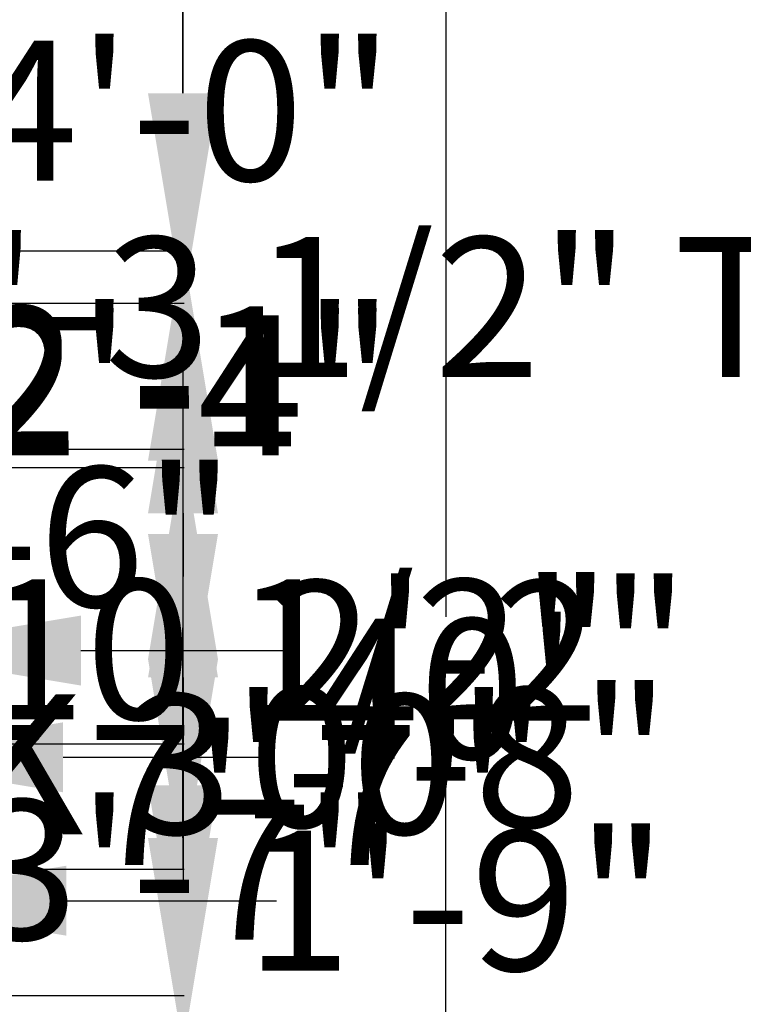
# Model space of a CAD drawing. Units: inches. Extents: x 2838 to 4029, y 1041 to 1915.
# Tile 11 of 16: x 3640 to 3764, y 1377 to 1546. Entities that reach past the tile are written whole.
import ezdxf

# ---------------------------------------------------------------- set-up
doc = ezdxf.new("R2010")
doc.units = ezdxf.units.IN
doc.header["$MEASUREMENT"] = 0
doc.layers.add('A-ANNO-DIMS', color=2, linetype='Continuous', lineweight=18)
doc.styles.get("Standard").update_dxf_attribs({"font": 'arial.ttf'})
doc.dimstyles.get("Standard").update_dxf_attribs({"dimtxt": 24, "dimasz": 36, "dimexe": 0.18, "dimexo": 0.0625, "dimgap": 0.09, "dimtad": 0, "dimtih": 1, "dimtoh": 1, "dimdec": 0, "dimzin": 0, "dimdsep": 46, "dimlunit": 3, "dimtxsty": 'Standard', "dimcen": 0.09, "dimadec": 0, "dimazin": 0, "dimtfac": 1, "dimtdec": 0, "dimtofl": 0, "dimtmove": 0, "dimatfit": 3, "dimfxl": 1, "dimtolj": 1, "dimtzin": 0, "dimarcsym": 0})

# ---------------------------------------------------------------- blocks, each defined once
blk = doc.blocks.new('*D17')
at = {"layer": 'A-ANNO-DIMS', "color": 0, "lineweight": -2, "transparency": 16777216}
for p, q in [((3627.79, 1671.3), (3713.18, 1671.3)), ((3713, 1635.3), (3713, 1443.64)), ((3713, 1227.3), (3713, 1418.95)), ((3627.79, 1191.3), (3713.18, 1191.3))]:
    blk.add_line(p, q, dxfattribs=at)
at = {"layer": 'A-ANNO-DIMS', "color": 0, "transparency": 16777216}
for points in [[(3707, 1635.3), (3719, 1635.3), (3713, 1671.3)], [(3707, 1227.3), (3719, 1227.3), (3713, 1191.3)]]:
    blk.add_solid(points, dxfattribs=at)
at = {"layer": 'Defpoints', "color": 0, "transparency": 16777216}
for p in [(3627.73, 1671.3), (3627.73, 1191.3), (3713, 1191.3)]:
    blk.add_point(p, dxfattribs=at)
at = {"layer": 'A-ANNO-DIMS', "color": 0, "transparency": 16777216, "insert": (3713, 1431.3), "char_height": 24, "attachment_point": 5}
blk.add_mtext("\\A1;40'", dxfattribs=at)
blk = doc.blocks.new('*D27')
at = {"layer": 'A-ANNO-DIMS', "color": 0, "lineweight": -2, "transparency": 16777216}
for p, q in [((3598.68, 1614.31), (3598.68, 1650.31)), ((3598.68, 1650.31), (3634.68, 1650.31)), ((3601.19, 1578.31), (3598.5, 1578.31)), ((3601.19, 1561.16), (3598.5, 1561.16)), ((3598.68, 1525.16), (3598.68, 1489.16))]:
    blk.add_line(p, q, dxfattribs=at)
at = {"layer": 'A-ANNO-DIMS', "color": 0, "transparency": 16777216}
for points in [[(3592.68, 1614.31), (3604.68, 1614.31), (3598.68, 1578.31)], [(3592.68, 1525.16), (3604.68, 1525.16), (3598.68, 1561.16)]]:
    blk.add_solid(points, dxfattribs=at)
at = {"layer": 'Defpoints', "color": 0, "transparency": 16777216}
for p in [(3598.68, 1578.31), (3601.25, 1578.31), (3601.25, 1561.16)]:
    blk.add_point(p, dxfattribs=at)
at = {"layer": 'A-ANNO-DIMS', "color": 0, "transparency": 16777216, "insert": (3820.96, 1650.31), "char_height": 24, "attachment_point": 5}
blk.add_mtext('\\A1;NIGHTSTAND 1\'-5" TYP.', dxfattribs=at)
blk = doc.blocks.new('*D28')
at = {"layer": 'A-ANNO-DIMS', "color": 0, "lineweight": -2, "transparency": 16777216}
for p, q in [((3565.25, 1580.88), (3529.25, 1580.88)), ((3601.25, 1578.37), (3601.25, 1581.06)), ((3617.82, 1578.37), (3617.82, 1581.06)), ((3653.82, 1580.88), (3689.82, 1580.88))]:
    blk.add_line(p, q, dxfattribs=at)
at = {"layer": 'A-ANNO-DIMS', "color": 0, "transparency": 16777216}
for points in [[(3565.25, 1586.88), (3565.25, 1574.88), (3601.25, 1580.88)], [(3653.82, 1586.88), (3653.82, 1574.88), (3617.82, 1580.88)]]:
    blk.add_solid(points, dxfattribs=at)
at = {"layer": 'Defpoints', "color": 0, "transparency": 16777216}
for p in [(3617.82, 1580.88), (3601.25, 1578.31), (3617.82, 1578.31)]:
    blk.add_point(p, dxfattribs=at)
at = {"layer": 'A-ANNO-DIMS', "color": 0, "transparency": 16777216, "insert": (3789.89, 1580.88), "char_height": 24, "attachment_point": 5}
blk.add_mtext('\\A1;1\'-4 1/2" TYP.', dxfattribs=at)
blk = doc.blocks.new('*D34')
at = {"layer": 'A-ANNO-DIMS', "color": 0, "lineweight": -2, "transparency": 16777216}
for p, q in [((3603.54, 1421.31), (3603.54, 1419.38)), ((3611.39, 1421.31), (3611.39, 1419.38)), ((3567.54, 1419.56), (3531.54, 1419.56)), ((3647.39, 1419.56), (3683.39, 1419.56))]:
    blk.add_line(p, q, dxfattribs=at)
at = {"layer": 'A-ANNO-DIMS', "color": 0, "transparency": 16777216}
for points in [[(3567.54, 1425.56), (3567.54, 1413.56), (3603.54, 1419.56)], [(3647.39, 1425.56), (3647.39, 1413.56), (3611.39, 1419.56)]]:
    blk.add_solid(points, dxfattribs=at)
at = {"layer": 'Defpoints', "color": 0, "transparency": 16777216}
for p in [(3603.54, 1421.37), (3611.39, 1421.37), (3611.39, 1419.56)]:
    blk.add_point(p, dxfattribs=at)
at = {"layer": 'A-ANNO-DIMS', "color": 0, "transparency": 16777216, "insert": (3715.38, 1419.56), "char_height": 24, "attachment_point": 5}
blk.add_mtext('\\A1;0\'-8"', dxfattribs=at)
blk = doc.blocks.new('*D41')
at = {"layer": 'A-ANNO-DIMS', "color": 0, "lineweight": -2, "transparency": 16777216}
for p, q in [((3284.24, 1506.2), (3284.24, 1496.56)), ((3347.73, 1506.2), (3347.73, 1496.56)), ((3248.24, 1496.74), (3212.24, 1496.74)), ((3383.73, 1496.74), (3419.73, 1496.74))]:
    blk.add_line(p, q, dxfattribs=at)
at = {"layer": 'A-ANNO-DIMS', "color": 0, "transparency": 16777216}
for points in [[(3248.24, 1502.74), (3248.24, 1490.74), (3284.24, 1496.74)], [(3383.73, 1502.74), (3383.73, 1490.74), (3347.73, 1496.74)]]:
    blk.add_solid(points, dxfattribs=at)
at = {"layer": 'Defpoints', "color": 0, "transparency": 16777216}
for p in [(3284.24, 1506.26), (3347.73, 1506.26), (3347.73, 1496.74)]:
    blk.add_point(p, dxfattribs=at)
at = {"layer": 'A-ANNO-DIMS', "color": 0, "transparency": 16777216, "insert": (3624.81, 1496.74), "char_height": 24, "attachment_point": 5}
blk.add_mtext('\\A1;WARDROBE 5\'-3 1/2" TYP.', dxfattribs=at)
blk = doc.blocks.new('*D47')
at = {"layer": 'A-ANNO-DIMS', "color": 0, "lineweight": -2, "transparency": 16777216}
for p, q in [((3493.47, 1640.5), (3493.47, 1676.5)), ((3493.47, 1676.5), (3529.47, 1676.5)), ((3489.85, 1604.5), (3493.65, 1604.5)), ((3489.85, 1579.95), (3493.65, 1579.95)), ((3493.47, 1543.95), (3493.47, 1507.95))]:
    blk.add_line(p, q, dxfattribs=at)
at = {"layer": 'A-ANNO-DIMS', "color": 0, "transparency": 16777216}
for points in [[(3487.47, 1640.5), (3499.47, 1640.5), (3493.47, 1604.5)], [(3487.47, 1543.95), (3499.47, 1543.95), (3493.47, 1579.95)]]:
    blk.add_solid(points, dxfattribs=at)
at = {"layer": 'Defpoints', "color": 0, "transparency": 16777216}
for p in [(3489.78, 1604.5), (3493.47, 1604.5), (3489.78, 1579.95)]:
    blk.add_point(p, dxfattribs=at)
at = {"layer": 'A-ANNO-DIMS', "color": 0, "transparency": 16777216, "insert": (3643.85, 1676.5), "char_height": 24, "attachment_point": 5}
blk.add_mtext('\\A1;BASIN 2\'-0 1/2"', dxfattribs=at)
blk = doc.blocks.new('*D49')
at = {"layer": 'A-ANNO-DIMS', "color": 0, "lineweight": -2, "transparency": 16777216}
for p, q in [((3336.37, 1426.68), (3336.37, 1412.92)), ((3427.37, 1426.68), (3427.37, 1412.92)), ((3372.37, 1413.1), (3391.37, 1413.1)), ((3427.37, 1413.1), (3463.37, 1413.1))]:
    blk.add_line(p, q, dxfattribs=at)
at = {"layer": 'A-ANNO-DIMS', "color": 0, "transparency": 16777216}
for points in [[(3372.37, 1419.1), (3372.37, 1407.1), (3336.37, 1413.1)], [(3391.37, 1419.1), (3391.37, 1407.1), (3427.37, 1413.1)]]:
    blk.add_solid(points, dxfattribs=at)
at = {"layer": 'Defpoints', "color": 0, "transparency": 16777216}
for p in [(3336.37, 1426.75), (3427.37, 1426.75), (3427.37, 1413.1)]:
    blk.add_point(p, dxfattribs=at)
at = {"layer": 'A-ANNO-DIMS', "color": 0, "transparency": 16777216, "insert": (3595.36, 1413.1), "char_height": 24, "attachment_point": 5}
blk.add_mtext('\\A1;DINING SET 7\'-7"', dxfattribs=at)
blk = doc.blocks.new('*D53')
at = {"layer": 'A-ANNO-DIMS', "color": 0, "lineweight": -2, "transparency": 16777216}
for p, q in [((3583.96, 1508.36), (3583.96, 1544.36)), ((3588.4, 1472.36), (3583.78, 1472.36)), ((3588.4, 1442.36), (3583.78, 1442.36)), ((3583.96, 1406.36), (3583.96, 1370.36))]:
    blk.add_line(p, q, dxfattribs=at)
at = {"layer": 'A-ANNO-DIMS', "color": 0, "transparency": 16777216}
for points in [[(3577.96, 1508.36), (3589.96, 1508.36), (3583.96, 1472.36)], [(3577.96, 1406.36), (3589.96, 1406.36), (3583.96, 1442.36)]]:
    blk.add_solid(points, dxfattribs=at)
at = {"layer": 'Defpoints', "color": 0, "transparency": 16777216}
for p in [(3588.46, 1472.36), (3583.96, 1442.36), (3588.46, 1442.36)]:
    blk.add_point(p, dxfattribs=at)
at = {"layer": 'A-ANNO-DIMS', "color": 0, "transparency": 16777216, "insert": (3583.96, 1457.36), "char_height": 24, "attachment_point": 5}
blk.add_mtext('\\A1;RANGE 2\'-6"', dxfattribs=at)
blk = doc.blocks.new('*D54')
at = {"layer": 'A-ANNO-DIMS', "color": 0, "lineweight": -2, "transparency": 16777216}
for p, q in [((3588.46, 1442.29), (3588.46, 1437.68)), ((3614.46, 1442.29), (3614.46, 1437.68)), ((3552.46, 1437.86), (3516.46, 1437.86)), ((3650.46, 1437.86), (3686.46, 1437.86))]:
    blk.add_line(p, q, dxfattribs=at)
at = {"layer": 'A-ANNO-DIMS', "color": 0, "transparency": 16777216}
for points in [[(3552.46, 1443.86), (3552.46, 1431.86), (3588.46, 1437.86)], [(3650.46, 1443.86), (3650.46, 1431.86), (3614.46, 1437.86)]]:
    blk.add_solid(points, dxfattribs=at)
at = {"layer": 'Defpoints', "color": 0, "transparency": 16777216}
for p in [(3588.46, 1442.36), (3614.46, 1442.36), (3614.46, 1437.86)]:
    blk.add_point(p, dxfattribs=at)
at = {"layer": 'A-ANNO-DIMS', "color": 0, "transparency": 16777216, "insert": (3718.65, 1437.86), "char_height": 24, "attachment_point": 5}
blk.add_mtext('\\A1;2\'-2"', dxfattribs=at)
blk = doc.blocks.new('*D56')
at = {"layer": 'A-ANNO-DIMS', "color": 0, "lineweight": -2, "transparency": 16777216}
for p, q in [((3567.44, 1530.6), (3567.44, 1566.6)), ((3567.44, 1566.6), (3603.44, 1566.6)), ((3562.33, 1494.6), (3567.62, 1494.6)), ((3562.33, 1470.6), (3567.62, 1470.6)), ((3567.44, 1434.6), (3567.44, 1398.6))]:
    blk.add_line(p, q, dxfattribs=at)
at = {"layer": 'A-ANNO-DIMS', "color": 0, "transparency": 16777216}
for points in [[(3561.44, 1530.6), (3573.44, 1530.6), (3567.44, 1494.6)], [(3561.44, 1434.6), (3573.44, 1434.6), (3567.44, 1470.6)]]:
    blk.add_solid(points, dxfattribs=at)
at = {"layer": 'Defpoints', "color": 0, "transparency": 16777216}
for p in [(3562.26, 1494.6), (3567.44, 1494.6), (3562.26, 1470.6)]:
    blk.add_point(p, dxfattribs=at)
at = {"layer": 'A-ANNO-DIMS', "color": 0, "transparency": 16777216, "insert": (3635.63, 1566.6), "char_height": 24, "attachment_point": 5}
blk.add_mtext('\\A1;2\'-0"', dxfattribs=at)
blk = doc.blocks.new('*D57')
at = {"layer": 'A-ANNO-DIMS', "color": 0, "lineweight": -2, "transparency": 16777216}
for p, q in [((3585.57, 1472.38), (3585.57, 1508.38)), ((3590.9, 1436.38), (3585.39, 1436.38)), ((3590.9, 1400.38), (3585.39, 1400.38)), ((3585.57, 1364.38), (3585.57, 1328.38))]:
    blk.add_line(p, q, dxfattribs=at)
at = {"layer": 'A-ANNO-DIMS', "color": 0, "transparency": 16777216}
for points in [[(3579.57, 1472.38), (3591.57, 1472.38), (3585.57, 1436.38)], [(3579.57, 1364.38), (3591.57, 1364.38), (3585.57, 1400.38)]]:
    blk.add_solid(points, dxfattribs=at)
at = {"layer": 'Defpoints', "color": 0, "transparency": 16777216}
for p in [(3590.97, 1436.38), (3585.57, 1400.38), (3590.97, 1400.38)]:
    blk.add_point(p, dxfattribs=at)
at = {"layer": 'A-ANNO-DIMS', "color": 0, "transparency": 16777216, "insert": (3585.57, 1418.38), "char_height": 24, "attachment_point": 5}
blk.add_mtext('\\A1;DOUBLE SINK 3\'-0"', dxfattribs=at)
blk = doc.blocks.new('*D58')
at = {"layer": 'A-ANNO-DIMS', "color": 0, "lineweight": -2, "transparency": 16777216}
for p, q in [((3590.97, 1400.32), (3590.97, 1394.8)), ((3611.97, 1400.32), (3611.97, 1394.8)), ((3554.97, 1394.98), (3518.97, 1394.98)), ((3647.97, 1394.98), (3683.97, 1394.98))]:
    blk.add_line(p, q, dxfattribs=at)
at = {"layer": 'A-ANNO-DIMS', "color": 0, "transparency": 16777216}
for points in [[(3554.97, 1400.98), (3554.97, 1388.98), (3590.97, 1394.98)], [(3647.97, 1400.98), (3647.97, 1388.98), (3611.97, 1394.98)]]:
    blk.add_solid(points, dxfattribs=at)
at = {"layer": 'Defpoints', "color": 0, "transparency": 16777216}
for p in [(3590.97, 1400.38), (3611.97, 1400.38), (3611.97, 1394.98)]:
    blk.add_point(p, dxfattribs=at)
at = {"layer": 'A-ANNO-DIMS', "color": 0, "transparency": 16777216, "insert": (3714.83, 1394.98), "char_height": 24, "attachment_point": 5}
blk.add_mtext('\\A1;1\'-9"', dxfattribs=at)
blk = doc.blocks.new('*D73')
at = {"layer": 'A-ANNO-DIMS', "color": 0, "lineweight": -2, "transparency": 16777216}
for p, q in [((3461.038746, 1200.359846), (3461.038746, 1711.702346)), ((3618.731626, 1200.359846), (3618.731626, 1711.702346)), ((3425.038746, 1711.522346), (3389.038746, 1711.522346)), ((3654.731626, 1711.522346), (3690.731626, 1711.522346))]:
    blk.add_line(p, q, dxfattribs=at)
at = {"layer": 'A-ANNO-DIMS', "color": 0, "transparency": 16777216}
for points in [[(3425.038746, 1717.522346), (3425.038746, 1705.522346), (3461.038746, 1711.522346)], [(3654.731626, 1717.522346), (3654.731626, 1705.522346), (3618.731626, 1711.522346)]]:
    blk.add_solid(points, dxfattribs=at)
at = {"layer": 'Defpoints', "color": 0, "transparency": 16777216}
for p in [(3618.731626, 1711.522346), (3461.038746, 1200.297346), (3618.731626, 1200.297346)]:
    blk.add_point(p, dxfattribs=at)
at = {"layer": 'A-ANNO-DIMS', "color": 0, "transparency": 16777216, "insert": (3539.885186, 1711.522346), "char_height": 24, "attachment_point": 5}
blk.add_mtext('\\A1;13\'-1 1/2"', dxfattribs=at)
blk = doc.blocks.new('*D75')
at = {"layer": 'A-ANNO-DIMS', "color": 0, "lineweight": -2, "transparency": 16777216}
for p, q in [((3667.956626, 1405.727214), (3667.956626, 1441.727214)), ((3618.794126, 1369.727214), (3668.136626, 1369.727214)), ((3618.794126, 1333.727214), (3668.136626, 1333.727214)), ((3667.956626, 1297.727214), (3667.956626, 1261.727214))]:
    blk.add_line(p, q, dxfattribs=at)
at = {"layer": 'A-ANNO-DIMS', "color": 0, "transparency": 16777216}
for points in [[(3661.956626, 1405.727214), (3673.956626, 1405.727214), (3667.956626, 1369.727214)], [(3661.956626, 1297.727214), (3673.956626, 1297.727214), (3667.956626, 1333.727214)]]:
    blk.add_solid(points, dxfattribs=at)
at = {"layer": 'Defpoints', "color": 0, "transparency": 16777216}
for p in [(3618.731626, 1369.727214), (3667.956626, 1369.727214), (3618.731626, 1333.727214)]:
    blk.add_point(p, dxfattribs=at)
at = {"layer": 'A-ANNO-DIMS', "color": 0, "transparency": 16777216, "insert": (3667.956626, 1351.727214), "char_height": 24, "attachment_point": 5}
blk.add_mtext('\\A1;3\'-0"', dxfattribs=at)
blk = doc.blocks.new('*D78')
at = {"layer": 'A-ANNO-DIMS', "color": 0, "lineweight": -2, "transparency": 16777216}
for p, q in [((3667.956626, 1590.394218), (3667.956626, 1626.394218)), ((3498.794126, 1554.394218), (3668.136626, 1554.394218)), ((3498.638013, 1506.394218), (3668.136626, 1506.394218)), ((3667.956626, 1470.394218), (3667.956626, 1434.394218))]:
    blk.add_line(p, q, dxfattribs=at)
at = {"layer": 'A-ANNO-DIMS', "color": 0, "transparency": 16777216}
for points in [[(3661.956626, 1590.394218), (3673.956626, 1590.394218), (3667.956626, 1554.394218)], [(3661.956626, 1470.394218), (3673.956626, 1470.394218), (3667.956626, 1506.394218)]]:
    blk.add_solid(points, dxfattribs=at)
at = {"layer": 'Defpoints', "color": 0, "transparency": 16777216}
for p in [(3498.731626, 1554.394218), (3667.956626, 1554.394218), (3498.575513, 1506.394218)]:
    blk.add_point(p, dxfattribs=at)
at = {"layer": 'A-ANNO-DIMS', "color": 0, "transparency": 16777216, "insert": (3667.956626, 1530.394218), "char_height": 24, "attachment_point": 5}
blk.add_mtext('\\A1;4\'-0"', dxfattribs=at)
blk = doc.blocks.new('*D88')
at = {"layer": 'A-ANNO-DIMS', "color": 0, "lineweight": -2, "transparency": 16777216}
for p, q in [((3522.73, 1378.66), (3522.73, 1081.89)), ((3618.73, 1378.66), (3618.73, 1081.89)), ((3558.73, 1082.07), (3582.73, 1082.07)), ((3618.73, 1082.07), (3654.73, 1082.07))]:
    blk.add_line(p, q, dxfattribs=at)
at = {"layer": 'A-ANNO-DIMS', "color": 0, "transparency": 16777216}
for points in [[(3558.73, 1088.07), (3558.73, 1076.07), (3522.73, 1082.07)], [(3582.73, 1088.07), (3582.73, 1076.07), (3618.73, 1082.07)]]:
    blk.add_solid(points, dxfattribs=at)
at = {"layer": 'Defpoints', "color": 0, "transparency": 16777216}
for p in [(3522.73, 1378.73), (3618.73, 1378.73), (3618.73, 1082.07)]:
    blk.add_point(p, dxfattribs=at)
at = {"layer": 'A-ANNO-DIMS', "color": 0, "transparency": 16777216, "insert": (3686.74, 1082.07), "char_height": 24, "attachment_point": 5}
blk.add_mtext('\\A1;8\'-0"', dxfattribs=at)
blk = doc.blocks.new('*D89')
at = {"layer": 'A-ANNO-DIMS', "color": 0, "lineweight": -2, "transparency": 16777216}
for p, q in [((3618.79, 1497.39), (3668.14, 1497.39)), ((3667.96, 1461.39), (3667.96, 1450.56)), ((3667.96, 1414.73), (3667.96, 1425.56)), ((3618.79, 1378.73), (3668.14, 1378.73))]:
    blk.add_line(p, q, dxfattribs=at)
at = {"layer": 'A-ANNO-DIMS', "color": 0, "transparency": 16777216}
for points in [[(3661.96, 1461.39), (3673.96, 1461.39), (3667.96, 1497.39)], [(3661.96, 1414.73), (3673.96, 1414.73), (3667.96, 1378.73)]]:
    blk.add_solid(points, dxfattribs=at)
at = {"layer": 'Defpoints', "color": 0, "transparency": 16777216}
for p in [(3618.73, 1497.39), (3667.96, 1497.39), (3618.73, 1378.73)]:
    blk.add_point(p, dxfattribs=at)
at = {"layer": 'A-ANNO-DIMS', "color": 0, "transparency": 16777216, "insert": (3667.96, 1438.06), "char_height": 24, "attachment_point": 5}
blk.add_mtext('\\A1;9\'-10 1/2"', dxfattribs=at)
blk = doc.blocks.new('*D90')
at = {"layer": 'A-ANNO-DIMS', "color": 0, "lineweight": -2, "transparency": 16777216}
for p, q in [((3667.96, 1457.85), (3667.96, 1493.85)), ((3618.79, 1421.85), (3668.14, 1421.85)), ((3618.79, 1378.73), (3668.14, 1378.73)), ((3667.96, 1342.73), (3667.96, 1306.73))]:
    blk.add_line(p, q, dxfattribs=at)
at = {"layer": 'A-ANNO-DIMS', "color": 0, "transparency": 16777216}
for points in [[(3661.96, 1457.85), (3673.96, 1457.85), (3667.96, 1421.85)], [(3661.96, 1342.73), (3673.96, 1342.73), (3667.96, 1378.73)]]:
    blk.add_solid(points, dxfattribs=at)
at = {"layer": 'Defpoints', "color": 0, "transparency": 16777216}
for p in [(3618.73, 1421.85), (3667.96, 1421.85), (3618.73, 1378.73)]:
    blk.add_point(p, dxfattribs=at)
at = {"layer": 'A-ANNO-DIMS', "color": 0, "transparency": 16777216, "insert": (3667.96, 1400.29), "char_height": 24, "attachment_point": 5}
blk.add_mtext('\\A1;3\'-7"', dxfattribs=at)
blk = doc.blocks.new('*D92')
at = {"layer": 'A-ANNO-DIMS', "color": 0, "lineweight": -2, "transparency": 16777216}
for p, q in [((3585.37, 1402), (3585.37, 1081.89)), ((3618.73, 1378.66), (3618.73, 1081.89)), ((3549.37, 1082.07), (3513.37, 1082.07)), ((3654.73, 1082.07), (3690.73, 1082.07))]:
    blk.add_line(p, q, dxfattribs=at)
at = {"layer": 'A-ANNO-DIMS', "color": 0, "transparency": 16777216}
for points in [[(3549.37, 1088.07), (3549.37, 1076.07), (3585.37, 1082.07)], [(3654.73, 1088.07), (3654.73, 1076.07), (3618.73, 1082.07)]]:
    blk.add_solid(points, dxfattribs=at)
at = {"layer": 'Defpoints', "color": 0, "transparency": 16777216}
for p in [(3585.37, 1402.06), (3618.73, 1378.73), (3618.73, 1082.07)]:
    blk.add_point(p, dxfattribs=at)
at = {"layer": 'A-ANNO-DIMS', "color": 0, "transparency": 16777216, "insert": (3750.89, 1082.07), "char_height": 24, "attachment_point": 5}
blk.add_mtext('\\A1;2\'-9 1/2"', dxfattribs=at)
blk = doc.blocks.new('*D94')
at = {"layer": 'A-ANNO-DIMS', "color": 0, "lineweight": -2, "transparency": 16777216}
for p, q in [((3667.96, 1533.39), (3667.96, 1569.39)), ((3585.44, 1497.39), (3668.14, 1497.39)), ((3585.44, 1469.25), (3668.14, 1469.25)), ((3667.96, 1433.25), (3667.96, 1397.25))]:
    blk.add_line(p, q, dxfattribs=at)
at = {"layer": 'A-ANNO-DIMS', "color": 0, "transparency": 16777216}
for points in [[(3661.96, 1533.39), (3673.96, 1533.39), (3667.96, 1497.39)], [(3661.96, 1433.25), (3673.96, 1433.25), (3667.96, 1469.25)]]:
    blk.add_solid(points, dxfattribs=at)
at = {"layer": 'Defpoints', "color": 0, "transparency": 16777216}
for p in [(3585.37, 1497.39), (3585.37, 1469.25), (3667.96, 1469.25)]:
    blk.add_point(p, dxfattribs=at)
at = {"layer": 'A-ANNO-DIMS', "color": 0, "transparency": 16777216, "insert": (3667.96, 1483.32), "char_height": 24, "attachment_point": 5}
blk.add_mtext('\\A1;2\'-4"', dxfattribs=at)
blk = doc.blocks.new('*D104')
at = {"layer": 'A-ANNO-DIMS', "color": 0, "lineweight": -2, "transparency": 16777216}
for p, q in [((3667.956626, 1533.394218), (3667.956626, 1569.394218)), ((3618.794126, 1497.394218), (3668.136626, 1497.394218)), ((3614.522024, 1472.357294), (3668.136626, 1472.357294)), ((3667.956626, 1436.357294), (3667.956626, 1400.357294))]:
    blk.add_line(p, q, dxfattribs=at)
at = {"layer": 'A-ANNO-DIMS', "color": 0, "transparency": 16777216}
for points in [[(3661.956626, 1533.394218), (3673.956626, 1533.394218), (3667.956626, 1497.394218)], [(3661.956626, 1436.357294), (3673.956626, 1436.357294), (3667.956626, 1472.357294)]]:
    blk.add_solid(points, dxfattribs=at)
at = {"layer": 'Defpoints', "color": 0, "transparency": 16777216}
for p in [(3618.731626, 1497.394218), (3614.459524, 1472.357294), (3667.956626, 1472.357294)]:
    blk.add_point(p, dxfattribs=at)
at = {"layer": 'A-ANNO-DIMS', "color": 0, "transparency": 16777216, "insert": (3667.956626, 1484.875756), "char_height": 24, "attachment_point": 5}
blk.add_mtext('\\A1;2\'-1"', dxfattribs=at)
blk = doc.blocks.new('*D105')
at = {"layer": 'A-ANNO-DIMS', "color": 0, "lineweight": -2, "transparency": 16777216}
for p, q in [((3614.46, 1472.42), (3614.46, 1711.7)), ((3618.73, 1469.91), (3618.73, 1711.7)), ((3578.46, 1711.52), (3542.46, 1711.52)), ((3654.73, 1711.52), (3690.73, 1711.52))]:
    blk.add_line(p, q, dxfattribs=at)
at = {"layer": 'A-ANNO-DIMS', "color": 0, "transparency": 16777216}
for points in [[(3578.46, 1717.52), (3578.46, 1705.52), (3614.46, 1711.52)], [(3654.73, 1717.52), (3654.73, 1705.52), (3618.73, 1711.52)]]:
    blk.add_solid(points, dxfattribs=at)
at = {"layer": 'Defpoints', "color": 0, "transparency": 16777216}
for p in [(3618.73, 1711.52), (3614.46, 1472.36), (3618.73, 1469.85)]:
    blk.add_point(p, dxfattribs=at)
at = {"layer": 'A-ANNO-DIMS', "color": 0, "transparency": 16777216, "insert": (3750.68, 1711.52), "char_height": 24, "attachment_point": 5}
blk.add_mtext('\\A1;0\'-4 1/2"', dxfattribs=at)
blk = doc.blocks.new('*D106')
at = {"layer": 'A-ANNO-DIMS', "color": 0, "lineweight": -2, "transparency": 16777216}
for p, q in [((3611.97, 1401.82), (3611.97, 1081.89)), ((3618.73, 1378.66), (3618.73, 1081.89)), ((3575.97, 1082.07), (3539.97, 1082.07)), ((3654.73, 1082.07), (3690.73, 1082.07))]:
    blk.add_line(p, q, dxfattribs=at)
at = {"layer": 'A-ANNO-DIMS', "color": 0, "transparency": 16777216}
for points in [[(3575.97, 1088.07), (3575.97, 1076.07), (3611.97, 1082.07)], [(3654.73, 1088.07), (3654.73, 1076.07), (3618.73, 1082.07)]]:
    blk.add_solid(points, dxfattribs=at)
at = {"layer": 'Defpoints', "color": 0, "transparency": 16777216}
for p in [(3611.97, 1401.88), (3618.73, 1378.73), (3618.73, 1082.07)]:
    blk.add_point(p, dxfattribs=at)
at = {"layer": 'A-ANNO-DIMS', "color": 0, "transparency": 16777216, "insert": (3722.72, 1082.07), "char_height": 24, "attachment_point": 5}
blk.add_mtext('\\A1;0\'-7"', dxfattribs=at)
blk = doc.blocks.new('*D107')
at = {"layer": 'A-ANNO-DIMS', "color": 0, "lineweight": -2, "transparency": 16777216}
for p, q in [((3667.96, 1436.38), (3667.96, 1472.38)), ((3610.53, 1400.38), (3668.14, 1400.38)), ((3618.79, 1378.73), (3668.14, 1378.73)), ((3667.96, 1342.73), (3667.96, 1306.73)), ((3667.96, 1306.73), (3631.96, 1306.73))]:
    blk.add_line(p, q, dxfattribs=at)
at = {"layer": 'A-ANNO-DIMS', "color": 0, "transparency": 16777216}
for points in [[(3661.96, 1436.38), (3673.96, 1436.38), (3667.96, 1400.38)], [(3661.96, 1342.73), (3673.96, 1342.73), (3667.96, 1378.73)]]:
    blk.add_solid(points, dxfattribs=at)
at = {"layer": 'Defpoints', "color": 0, "transparency": 16777216}
for p in [(3610.47, 1400.38), (3618.73, 1378.73), (3667.96, 1378.73)]:
    blk.add_point(p, dxfattribs=at)
at = {"layer": 'A-ANNO-DIMS', "color": 0, "transparency": 16777216, "insert": (3573.14, 1306.73), "char_height": 24, "attachment_point": 5}
blk.add_mtext('\\A1;1\'-9 1/2"', dxfattribs=at)

msp = doc.modelspace()

# ---------------------------------------------------------------- dimensions: what is measured, and where the dimension line sits
at = {"layer": 'A-ANNO-DIMS'}
for base, p1, p2, picture, middle in [((3618.73, 1711.52), (3461.04, 1200.3), (3618.73, 1200.3), '*D73', (3539.89, 1711.52)), ((3618.73, 1711.52), (3614.46, 1472.36), (3618.73, 1469.85), '*D105', (3750.68, 1711.52)), ((3614.46, 1437.86), (3588.46, 1442.36), (3614.46, 1442.36), '*D54', (3718.65, 1437.86)), ((3611.3929, 1419.5634), (3603.5434, 1421.3748), (3611.3929, 1421.3748), '*D34', (3715.382, 1419.5634)), ((3611.97, 1394.98), (3590.97, 1400.38), (3611.97, 1400.38), '*D58', (3714.83, 1394.98)), ((3618.73, 1082.07), (3585.37, 1402.06), (3618.73, 1378.73), '*D92', (3750.89, 1082.07)), ((3618.73, 1082.07), (3611.97, 1401.88), (3618.73, 1378.73), '*D106', (3722.72, 1082.07)), ((3618.73, 1082.07), (3522.73, 1378.73), (3618.73, 1378.73), '*D88', (3686.74, 1082.07))]:
    dim = msp.add_linear_dim(base=base, p1=p1, p2=p2, dimstyle='Standard', override={"dimdec": 1, "dimlfac": 1, "dimrnd": 0, "dimzin": 1, "dimdsep": 46, "dimlunit": 4, "dimfrac": 2}, dxfattribs=at)
    dim.commit()
    dim.dimension.update_dxf_attribs({"geometry": picture, "text_midpoint": middle})
for base, p1, p2, angle, text, picture, middle in [((3493.4667, 1604.5013), (3489.7841, 1579.9504), (3489.7841, 1604.5013), 90, 'BASIN <>', '*D47', (3643.8514, 1676.5013)), ((3598.6826, 1578.3092), (3601.2549, 1561.1604), (3601.2549, 1578.3092), 90, 'NIGHTSTAND <> TYP.', '*D27', (3820.9609, 1650.3092)), ((3583.96, 1442.36), (3588.46, 1472.36), (3588.46, 1442.36), 270, 'RANGE <>', '*D53', (3583.96, 1457.36)), ((3585.57, 1400.38), (3590.97, 1436.38), (3590.97, 1400.38), 270, 'DOUBLE SINK <>', '*D57', (3585.57, 1418.38))]:
    dim = msp.add_linear_dim(base=base, p1=p1, p2=p2, angle=angle, text=text, dimstyle='Standard', override={"dimdec": 1, "dimlfac": 1, "dimrnd": 0, "dimzin": 1, "dimdsep": 46, "dimlunit": 4, "dimfrac": 2}, dxfattribs=at)
    dim.commit()
    dim.dimension.update_dxf_attribs({"geometry": picture, "text_midpoint": middle})
for base, p1, p2, override, picture, middle in [((3713, 1191.3), (3627.73, 1671.3), (3627.73, 1191.3), {"dimclrd": 0, "dimclre": 0, "dimclrt": 0}, '*D17', (3713, 1431.3)), ((3667.96, 1554.39), (3498.58, 1506.39), (3498.73, 1554.39), {"dimdec": 1, "dimlfac": 1, "dimrnd": 0, "dimzin": 1, "dimdsep": 46, "dimlunit": 4, "dimfrac": 2}, '*D78', (3667.96, 1530.39)), ((3567.44, 1494.6), (3562.26, 1470.6), (3562.26, 1494.6), {"dimdec": 1, "dimlfac": 1, "dimrnd": 0, "dimzin": 1, "dimdsep": 46, "dimlunit": 4, "dimfrac": 2}, '*D56', (3635.63, 1566.6)), ((3667.96, 1469.25), (3585.37, 1497.39), (3585.37, 1469.25), {"dimdec": 1, "dimlfac": 1, "dimrnd": 0, "dimzin": 1, "dimdsep": 46, "dimlunit": 4, "dimfrac": 2}, '*D94', (3667.96, 1483.32)), ((3667.96, 1472.36), (3618.73, 1497.39), (3614.46, 1472.36), {"dimdec": 1, "dimlfac": 1, "dimrnd": 0, "dimzin": 1, "dimdsep": 46, "dimlunit": 4, "dimfrac": 2}, '*D104', (3667.96, 1484.88)), ((3667.96, 1497.39), (3618.73, 1378.73), (3618.73, 1497.39), {"dimdec": 1, "dimlfac": 1, "dimrnd": 0, "dimzin": 1, "dimdsep": 46, "dimlunit": 4, "dimfrac": 2}, '*D89', (3667.96, 1438.06)), ((3667.96, 1421.85), (3618.73, 1378.73), (3618.73, 1421.85), {"dimdec": 1, "dimlfac": 1, "dimrnd": 0, "dimzin": 1, "dimdsep": 46, "dimlunit": 4, "dimfrac": 2}, '*D90', (3667.96, 1400.29)), ((3667.9566, 1378.7272), (3610.4672, 1400.3841), (3618.7316, 1378.7272), {"dimdec": 1, "dimlfac": 1, "dimrnd": 0, "dimzin": 1, "dimdsep": 46, "dimlunit": 4, "dimfrac": 2}, '*D107', (3573.1354, 1306.7272)), ((3667.96, 1369.73), (3618.73, 1333.73), (3618.73, 1369.73), {"dimdec": 1, "dimlfac": 1, "dimrnd": 0, "dimzin": 1, "dimdsep": 46, "dimlunit": 4, "dimfrac": 2}, '*D75', (3667.96, 1351.73))]:
    dim = msp.add_linear_dim(base=base, p1=p1, p2=p2, angle=90, dimstyle='Standard', override=override, dxfattribs=at)
    dim.commit()
    dim.dimension.update_dxf_attribs({"geometry": picture, "text_midpoint": middle})
for base, p1, p2, text, picture, middle in [((3617.82, 1580.88), (3601.25, 1578.31), (3617.82, 1578.31), '<> TYP.', '*D28', (3789.89, 1580.88)), ((3347.73, 1496.74), (3284.24, 1506.26), (3347.73, 1506.26), 'WARDROBE <> TYP.', '*D41', (3624.81, 1496.74)), ((3427.37, 1413.1), (3336.37, 1426.75), (3427.37, 1426.75), 'DINING SET <>', '*D49', (3595.36, 1413.1))]:
    dim = msp.add_linear_dim(base=base, p1=p1, p2=p2, text=text, dimstyle='Standard', override={"dimdec": 1, "dimlfac": 1, "dimrnd": 0, "dimzin": 1, "dimdsep": 46, "dimlunit": 4, "dimfrac": 2}, dxfattribs=at)
    dim.commit()
    dim.dimension.update_dxf_attribs({"geometry": picture, "text_midpoint": middle})

doc.saveas('drawing.dxf')
